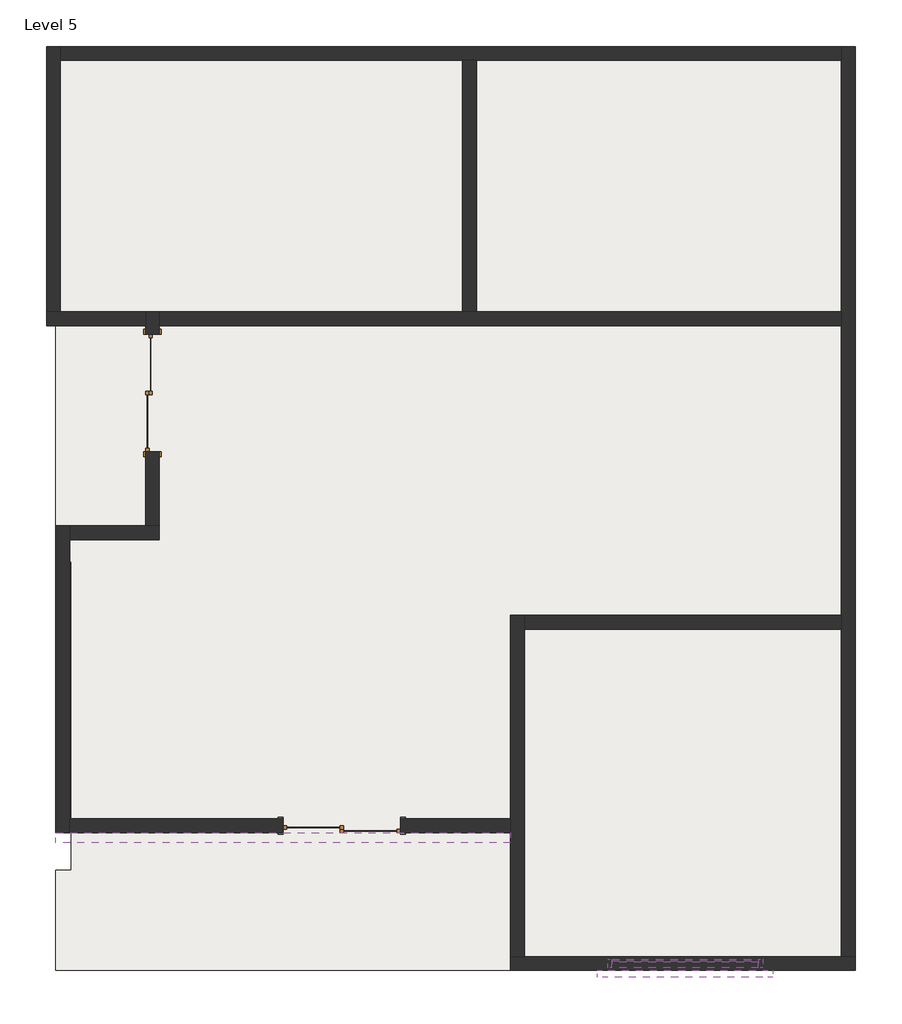
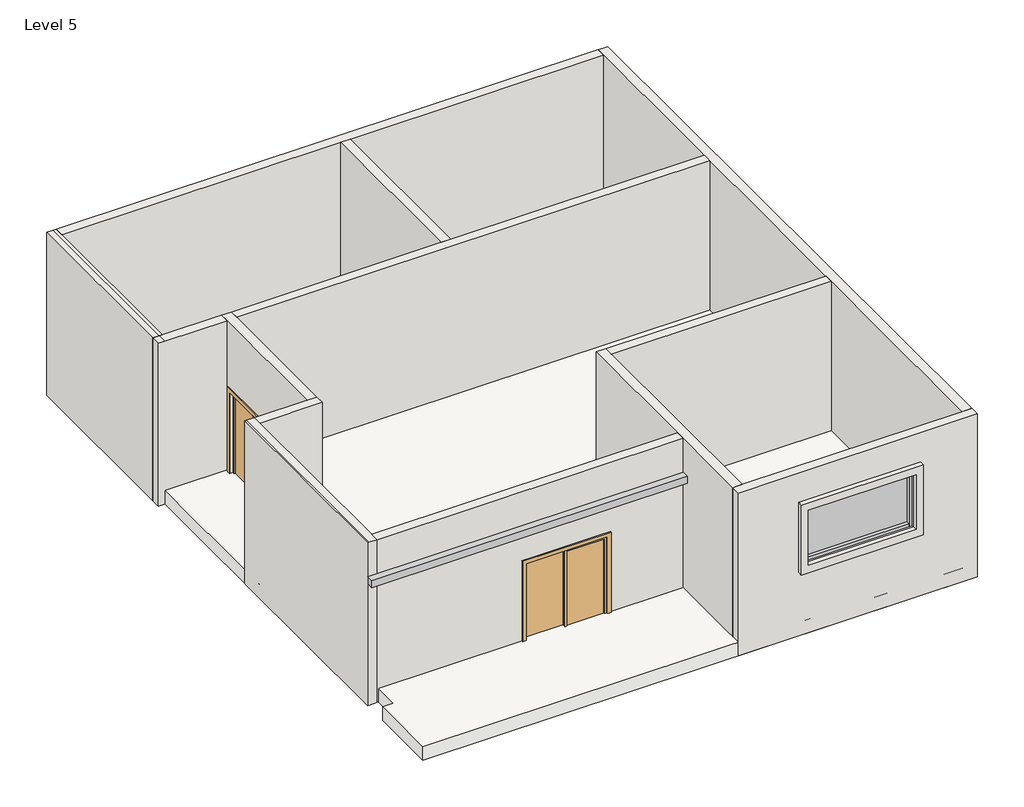
# One storey: 14 walls, 4 members, 2 doors, 1 plate, 1 proxy, 1 roof.
"""IFC4 building model written with IfcOpenShell, lengths in millimetres."""

from ifc_helpers import new_model, si_unit, frame, origin, place, context, project, spatial, polyline, outline, extrude, faceted_brep, transform, mapped, element, save
from components import door_076b30e0, member_3a6679d5, member_c08f7e50, system_panel_glazed_5a0db22b, walls_3_walls_1_a56c50be

model = new_model("IFC4")

# Units and contexts
model_context = context("Model", 3, world=origin())
ifc_project = project(units=[si_unit("LENGTHUNIT", "METRE", prefix="MILLI")], contexts=[model_context])

# Site, building, storey
site = spatial("IfcSite", under=ifc_project)
building = spatial("IfcBuilding", under=site)
storey = spatial("IfcBuildingStorey", under=building, Name="Level 5", Elevation=14630.4)

# Proxy
placement = place(None, origin())
element("IfcBuildingElementProxy", 1, Name="Cornice", ObjectType="Cornice", at=placement, inside=storey, context=model_context, shape_type="SweptSolid", body=[
    extrude(outline(polyline([(-8860.5727738, -2109.6325754), (-8860.5727738, -1957.2325754), (-2155.3436544, -1957.2325754), (-2155.3436544, -2109.6325754), (-8860.5727738, -2109.6325754)])), frame((0.0, 0.0, 17373.6), z_axis=(0.0, 0.0, 1.0), x_axis=(1.0, 0.0, 0.0)), (0.0, 0.0, 1.0), 152.4),
])

# Doors
door_shape = door_076b30e0(model_context)
element("IfcDoor", 2, ObjectType="Door-Double-Sliding : 68\" x 80\"", at=placement, inside=storey, context=model_context, shape_type="MappedRepresentation", body=[
    mapped(door_shape, transform((-7311.1727738, 4519.7674246, 14732.0), x_axis=(0.0, 1.0, 0.0), y_axis=(-1.0, 0.0, 0.0), z_axis=(0.0, 0.0, 1.0))),
])
element("IfcDoor", 3, ObjectType="Door-Double-Sliding : 68\" x 80\"", at=placement, inside=storey, context=model_context, shape_type="MappedRepresentation", body=[
    mapped(door_shape, transform((-4644.5436544, -1728.6325754, 14630.4), x_axis=(-1.0, 0.0, 0.0), y_axis=(0.0, -1.0, 0.0), z_axis=(0.0, 0.0, 1.0))),
])

# Members
member_shape = member_3a6679d5(model_context)
element("IfcMember", 4, ObjectType="Rectangular Mullion : 2.5\" x 5\" rectangular", at=placement, inside=storey, context=model_context, shape_type="MappedRepresentation", body=[
    mapped(member_shape, transform((1560.0533085, -3887.6325754, 16233.9422066), x_axis=(1.0, 0.0, 0.0), y_axis=(0.0, -1.0, 0.0), z_axis=(0.0, 0.0, -1.0))),
])
member_2_shape = member_c08f7e50(model_context)
element("IfcMember", 5, ObjectType="Rectangular Mullion : 2.5\" x 5\" rectangular", at=placement, inside=storey, context=model_context, shape_type="MappedRepresentation", body=[
    mapped(member_2_shape, transform((-662.4466915, -3887.6325754, 16233.9422066), x_axis=(0.0, 0.0, -1.0), y_axis=(0.0, -1.0, 0.0), z_axis=(-1.0, 0.0, 0.0))),
])
element("IfcMember", 6, ObjectType="Rectangular Mullion : 2.5\" x 5\" rectangular", at=placement, inside=storey, context=model_context, shape_type="MappedRepresentation", body=[
    mapped(member_2_shape, transform((1496.5533085, -3887.6325754, 17464.824337), x_axis=(0.0, 0.0, 1.0), y_axis=(0.0, -1.0, 0.0), z_axis=(1.0, 0.0, 0.0))),
])
element("IfcMember", 7, ObjectType="Rectangular Mullion : 2.5\" x 5\" rectangular", at=placement, inside=storey, context=model_context, shape_type="MappedRepresentation", body=[
    mapped(member_shape, transform((-725.9466915, -3887.6325754, 17464.824337), x_axis=(-1.0, 0.0, 0.0), y_axis=(0.0, -1.0, 0.0), z_axis=(0.0, 0.0, 1.0))),
])

# Plate
system_panel_glazed_shape = system_panel_glazed_5a0db22b(model_context)
element("IfcPlate", 8, ObjectType="System Panel : Glazed", at=placement, inside=storey, context=model_context, shape_type="MappedRepresentation", body=[
    mapped(system_panel_glazed_shape, transform((417.0533085, -3887.6325754, 16297.4422066), x_axis=(1.0, 0.0, 0.0), y_axis=(0.0, 1.0, 0.0), z_axis=(0.0, 0.0, 1.0))),
])

# Roof
element("IfcRoof", 9, ObjectType="Generic - 12\"", at=placement, inside=storey, context=model_context, shape_type="SweptSolid", body=[
    extrude(outline(polyline([(-8860.5727738, 9529.9174246), (2924.6563456, 9529.9174246), (2924.6563456, -3989.2325754), (-8860.5727738, -3989.2325754), (-8860.5727738, -2509.6825754), (-8631.9727738, -2509.6825754), (-8631.9727738, 2036.9174246), (-8860.5727738, 2036.9174246), (-8860.5727738, 9529.9174246)])), frame((0.0, 0.0, 14630.4), z_axis=(0.0, 0.0, 1.0), x_axis=(1.0, 0.0, 0.0)), (0.0, 0.0, 1.0), 304.8),
])

# Walls
element("IfcWall", 10, ObjectType="Generic - 8\"", at=placement, inside=storey, context=model_context, shape_type="Brep", body=[
    faceted_brep([(2924.6563456, -3786.0325754, 14630.4), (2721.4563456, -3786.0325754, 14630.4), (-1952.1436544, -3786.0325754, 14630.4), (-2155.3436544, -3786.0325754, 14630.4), (-2155.3436544, -3786.0325754, 18288.0), (-1952.1436544, -3786.0325754, 18288.0), (2721.4563456, -3786.0325754, 18288.0), (2924.6563456, -3786.0325754, 18288.0), (1560.0533085, -3786.0325754, 17464.824337), (-725.9466915, -3786.0325754, 17464.824337), (-725.9466915, -3786.0325754, 16233.9422066), (1560.0533085, -3786.0325754, 16233.9422066), (2924.6563456, -3989.2325754, 14630.4), (2924.6563456, -3989.2325754, 18288.0), (-2155.3436544, -3989.2325754, 18288.0), (-2155.3436544, -3989.2325754, 14630.4), (1560.0533085, -3989.2325754, 17464.824337), (1560.0533085, -3989.2325754, 16233.9422066), (-725.9466915, -3989.2325754, 16233.9422066), (-725.9466915, -3989.2325754, 17464.824337)], [[[0, 1, 2, 3, 4, 5, 6, 7], [8, 9, 10, 11]], [[12, 13, 14, 15], [16, 17, 18, 19]], [[4, 3, 15, 14]], [[0, 7, 13, 12]], [[3, 2, 1, 0, 12, 15]], [[9, 8, 16, 19]], [[10, 9, 19, 18]], [[11, 10, 18, 17]], [[8, 11, 17, 16]], [[7, 6, 5, 4, 14, 13]]]),
])
element("IfcWall", 11, ObjectType="Generic - 8\"", at=placement, inside=storey, context=model_context, shape_type="Brep", body=[
    faceted_brep([(-1952.1436544, -3786.0325754, 14630.4), (-1952.1436544, 1039.9674246, 14630.4), (-1952.1436544, 1243.1674246, 14630.4), (-1952.1436544, 1243.1674246, 18288.0), (-1952.1436544, 1039.9674246, 18288.0), (-1952.1436544, -3786.0325754, 18288.0), (-2155.3436544, -3786.0325754, 14630.4), (-2155.3436544, -3786.0325754, 18288.0), (-2155.3436544, -1957.2325754, 18288.0), (-2155.3436544, -1754.0325754, 18288.0), (-2155.3436544, 1243.1674246, 18288.0), (-2155.3436544, 1243.1674246, 14630.4), (-2155.3436544, -1754.0325754, 14630.4), (-2155.3436544, -1957.2325754, 14630.4)], [[[0, 1, 2, 3, 4, 5]], [[6, 7, 8, 9, 10, 11, 12, 13]], [[2, 1, 0, 6, 13, 12, 11]], [[0, 5, 7, 6]], [[3, 2, 11, 10]], [[5, 4, 3, 10, 9, 8, 7]]]),
])
element("IfcWall", 12, ObjectType="Generic - 8\"", at=placement, inside=storey, context=model_context, shape_type="SweptSolid", body=[
    extrude(outline(polyline([(2716.475018, 1039.9674246), (-1952.1436544, 1039.9674246), (-1952.1436544, 1243.1674246), (2716.475018, 1243.1674246), (2716.475018, 1039.9674246)])), frame((0.0, 0.0, 14630.4), z_axis=(0.0, 0.0, 1.0), x_axis=(1.0, 0.0, 0.0)), (0.0, 0.0, 1.0), 3657.6),
])
element("IfcWall", 13, ObjectType="Generic - 8\"", at=placement, inside=storey, context=model_context, shape_type="SweptSolid", body=[
    extrude(outline(polyline([(2924.6563456, 9625.1674246), (2924.6563456, -3786.0325754), (2721.4563456, -3786.0325754), (2721.4563456, 9625.1674246), (2924.6563456, 9625.1674246)])), frame((0.0, 0.0, 14630.4), z_axis=(0.0, 0.0, 1.0), x_axis=(1.0, 0.0, 0.0)), (0.0, 0.0, 1.0), 3657.6),
])
element("IfcWall", 14, ObjectType="Generic - 8\"", at=placement, inside=storey, context=model_context, shape_type="Brep", body=[
    faceted_brep([(-8657.3727738, -1957.2325754, 14630.4), (-8657.3727738, -1754.0325754, 14630.4), (-8657.3727738, 2360.7674246, 14630.4), (-8657.3727738, 2563.9674246, 14630.4), (-8657.3727738, 2563.9674246, 18288.0), (-8657.3727738, 2360.7674246, 18288.0), (-8657.3727738, -1754.0325754, 18288.0), (-8657.3727738, -1957.2325754, 18288.0), (-8860.5727738, -1957.2325754, 14630.4), (-8860.5727738, -1957.2325754, 18288.0), (-8860.5727738, 2563.9674246, 18288.0), (-8860.5727738, 2563.9674246, 14630.4), (-8835.1727738, 2563.9674246, 18288.0), (-8835.1727738, -1957.2325754, 18288.0)], [[[0, 1, 2, 3, 4, 5, 6, 7]], [[8, 9, 10, 11]], [[3, 2, 1, 0, 8, 11]], [[4, 3, 11, 10, 12]], [[0, 7, 13, 9, 8]], [[12, 10, 9, 13]], [[7, 6, 5, 4, 12, 13]]]),
])
element("IfcWall", 15, ObjectType="Generic - 8\"", at=placement, inside=storey, context=model_context, shape_type="Brep", body=[
    faceted_brep([(-8657.3727738, 2360.7674246, 14630.4), (-7336.5727738, 2360.7674246, 14630.4), (-7336.5727738, 2360.7674246, 18288.0), (-8657.3727738, 2360.7674246, 18288.0), (-8657.3727738, 2563.9674246, 14630.4), (-8657.3727738, 2563.9674246, 18288.0), (-7539.7727738, 2563.9674246, 18288.0), (-7336.5727738, 2563.9674246, 18288.0), (-7336.5727738, 2563.9674246, 14630.4), (-7539.7727738, 2563.9674246, 14630.4)], [[[0, 1, 2, 3]], [[4, 5, 6, 7, 8, 9]], [[1, 0, 4, 9, 8]], [[0, 3, 5, 4]], [[2, 1, 8, 7]], [[3, 2, 7, 6, 5]]]),
])
element("IfcWall", 16, ObjectType="Generic - 8\"", at=placement, inside=storey, context=model_context, shape_type="Brep", body=[
    faceted_brep([(-7336.5727738, 2563.9674246, 14630.4), (-7336.5727738, 5510.3674246, 14630.4), (-7336.5727738, 5713.5674246, 14630.4), (-7336.5727738, 5713.5674246, 18288.0), (-7336.5727738, 5510.3674246, 18288.0), (-7336.5727738, 2563.9674246, 18288.0), (-7336.5727738, 3656.1674246, 16764.0), (-7336.5727738, 5383.3674246, 16764.0), (-7336.5727738, 5383.3674246, 14732.0), (-7336.5727738, 3656.1674246, 14732.0), (-7539.7727738, 2563.9674246, 14630.4), (-7539.7727738, 2563.9674246, 18288.0), (-7539.7727738, 5510.3674246, 18288.0), (-7539.7727738, 5713.5674246, 18288.0), (-7539.7727738, 5713.5674246, 14630.4), (-7539.7727738, 5510.3674246, 14630.4), (-7539.7727738, 3656.1674246, 16764.0), (-7539.7727738, 3656.1674246, 14732.0), (-7539.7727738, 5383.3674246, 14732.0), (-7539.7727738, 5383.3674246, 16764.0)], [[[0, 1, 2, 3, 4, 5], [6, 7, 8, 9]], [[10, 11, 12, 13, 14, 15], [16, 17, 18, 19]], [[2, 1, 0, 10, 15, 14]], [[0, 5, 11, 10]], [[3, 2, 14, 13]], [[5, 4, 3, 13, 12, 11]], [[17, 16, 6, 9]], [[18, 17, 9, 8]], [[19, 18, 8, 7]], [[16, 19, 7, 6]]]),
])
element("IfcWall", 17, ObjectType="Generic - 8\"", at=placement, inside=storey, context=model_context, shape_type="Brep", body=[
    faceted_brep([(-7539.7727738, 5713.5674246, 14630.4), (-8796.074982, 5713.5674246, 14630.4), (-8999.274982, 5713.5674246, 14630.4), (-8999.274982, 5713.5674246, 18288.0), (-8860.5727738, 5713.5674246, 18288.0), (-8796.074982, 5713.5674246, 18288.0), (-7539.7727738, 5713.5674246, 18288.0), (-7539.7727738, 5510.3674246, 14630.4), (-7539.7727738, 5510.3674246, 18288.0), (-8860.5727738, 5510.3674246, 18288.0), (-8999.274982, 5510.3674246, 18288.0), (-8999.274982, 5510.3674246, 14630.4)], [[[0, 1, 2, 3, 4, 5, 6]], [[7, 8, 9, 10, 11]], [[2, 1, 0, 7, 11]], [[0, 6, 8, 7]], [[3, 2, 11, 10]], [[4, 3, 10, 9]], [[6, 5, 4, 9, 8]]]),
])
element("IfcWall", 18, ObjectType="Generic - 8\"", at=placement, inside=storey, context=model_context, shape_type="Brep", body=[
    faceted_brep([(-8796.074982, 5713.5674246, 14630.4), (-8796.074982, 9421.9674246, 14630.4), (-8796.074982, 9625.1674246, 14630.4), (-8796.074982, 9625.1674246, 18288.0), (-8796.074982, 9421.9674246, 18288.0), (-8796.074982, 5713.5674246, 18288.0), (-8999.274982, 5713.5674246, 14630.4), (-8999.274982, 5713.5674246, 18288.0), (-8999.274982, 9625.1674246, 18288.0), (-8999.274982, 9625.1674246, 14630.4), (-8860.5727738, 5713.5674246, 18288.0), (-8860.5727738, 9625.1674246, 18288.0)], [[[0, 1, 2, 3, 4, 5]], [[6, 7, 8, 9]], [[2, 1, 0, 6, 9]], [[0, 5, 10, 7, 6]], [[3, 2, 9, 8, 11]], [[5, 4, 3, 11, 10]], [[11, 8, 7, 10]]]),
])
element("IfcWall", 19, ObjectType="Generic - 8\"", at=placement, inside=storey, context=model_context, shape_type="Brep", body=[
    faceted_brep([(-8796.074982, 9421.9674246, 14630.4), (-2866.5436544, 9421.9674246, 14630.4), (-2663.3436544, 9421.9674246, 14630.4), (2716.475018, 9421.9674246, 14630.4), (2716.475018, 9421.9674246, 18288.0), (-2663.3436544, 9421.9674246, 18288.0), (-2866.5436544, 9421.9674246, 18288.0), (-8796.074982, 9421.9674246, 18288.0), (-8796.074982, 9625.1674246, 14630.4), (-8796.074982, 9625.1674246, 18288.0), (2716.475018, 9625.1674246, 18288.0), (2716.475018, 9625.1674246, 14630.4)], [[[0, 1, 2, 3, 4, 5, 6, 7]], [[8, 9, 10, 11]], [[3, 2, 1, 0, 8, 11]], [[4, 3, 11, 10]], [[0, 7, 9, 8]], [[7, 6, 5, 4, 10, 9]]]),
])
element("IfcWall", 20, ObjectType="Generic - 8\"", at=placement, inside=storey, context=model_context, shape_type="Brep", body=[
    faceted_brep([(-7336.5727738, 5510.3674246, 14630.4), (2716.475018, 5510.3674246, 14630.4), (2716.475018, 5510.3674246, 18288.0), (-7336.5727738, 5510.3674246, 18288.0), (-7336.5727738, 5713.5674246, 14630.4), (-7336.5727738, 5713.5674246, 18288.0), (-2866.5436544, 5713.5674246, 18288.0), (-2663.3436544, 5713.5674246, 18288.0), (2716.475018, 5713.5674246, 18288.0), (2716.475018, 5713.5674246, 14630.4), (-2663.3436544, 5713.5674246, 14630.4), (-2866.5436544, 5713.5674246, 14630.4)], [[[0, 1, 2, 3]], [[4, 5, 6, 7, 8, 9, 10, 11]], [[1, 0, 4, 11, 10, 9]], [[2, 1, 9, 8]], [[0, 3, 5, 4]], [[3, 2, 8, 7, 6, 5]]]),
])
element("IfcWall", 21, ObjectType="Generic - 8\"", at=placement, inside=storey, context=model_context, shape_type="SweptSolid", body=[
    extrude(outline(polyline([(-2663.3436544, 9421.9674246), (-2663.3436544, 5713.5674246), (-2866.5436544, 5713.5674246), (-2866.5436544, 9421.9674246), (-2663.3436544, 9421.9674246)])), frame((0.0, 0.0, 14630.4), z_axis=(0.0, 0.0, 1.0), x_axis=(1.0, 0.0, 0.0)), (0.0, 0.0, 1.0), 3657.6),
])
element("IfcWall", 22, ObjectType="Generic - 8\"", at=placement, inside=storey, context=model_context, shape_type="SweptSolid", body=[
    extrude(outline(polyline([(14630.4, -8657.3727738), (14630.4, -5508.1436544), (16662.4, -5508.1436544), (16662.4, -3780.9436544), (14630.4, -3780.9436544), (14630.4, -2155.3436544), (18288.0, -2155.3436544), (18288.0, -8657.3727738), (14630.4, -8657.3727738)])), frame((0.0, -1957.2325754, 0.0), z_axis=(0.0, 1.0, 0.0), x_axis=(0.0, 0.0, 1.0)), (0.0, 0.0, 1.0), 203.2),
])
walls_3_walls_1_shape = walls_3_walls_1_a56c50be(model_context)
element("IfcWall", 23, ObjectType="Walls 3 : Walls 1", at=placement, inside=storey, context=model_context, shape_type="MappedRepresentation", body=[
    mapped(walls_3_walls_1_shape, transform((0.0, 0.0, 0.0), x_axis=(1.0, 0.0, 0.0), y_axis=(0.0, 1.0, 0.0), z_axis=(0.0, 0.0, 1.0))),
])

save(model, "model.ifc")

# Revit data of these elements
# Type "Door-Double-Sliding : 68\" x 80\""
#   Type Mark = "10"
#   Construction Type Id = "opn-d45"
#   Assembly Code = "C1020"
#   Analytic Construction = "Wood frame, double glass door "
#   Thickness = 0' - 2"
#   Thermal Resistance (R) = 1.8150 (h·ft²·°F)/BTU
#   Heat Transfer Coefficient (U) = 0.5510 BTU/(h·ft²·°F)
#   Height = 6' - 8"
#   Rail Width = 0' - 2"
#   Stiles = 0' - 2"
#   Trim Projection Ext = 0' - 1"
#   Trim Projection Int = 0' - 1"
#   Trim Width = 0' - 3"
#   Width = 5' - 8"
#   Define Thermal Properties by = 1
#   Glazing = Glass
#   Panel Material = Wood - Birch - Solid Stained Light Low Gloss
#   Trim Material = Paint - Sienna
#   Visual Light Transmittance = 0
#   Solar Heat Gain Coefficient = 0
#   Function = (empty or 0)
#   Wall Closure = (empty or 0)
# Type "Rectangular Mullion : 2.5\" x 5\" rectangular"
#   built-in parameter 1007304 = 0.416667 (stored number, unit not read)
#   built-in parameter 1007301 = 0.104167 (stored number, unit not read)
#   built-in parameter 1007300 = 0.104167 (stored number, unit not read)
# Type "System Panel : Glazed"
#   Construction Type Id = "GSP4R"
#   Analytic Construction = "1/8 in Pilkington single glazing"
#   Visual Light Transmittance = 0.9
#   Solar Heat Gain Coefficient = 0.86
#   Heat Transfer Coefficient (U) = 1.18115 BTU/(h·ft²·°F)
# Type "Generic - 12\""
#   Assembly Code = "B1020"
#   Layers, outside or top first: 1' - 0" no material (function 1)
# Type "Generic - 8\""
#   Assembly Code = "B2010"
#   Layers, outside or top first: 0' - 8" no material (function 1)
# Element 1 (IfcBuildingElementProxy, "Cornice")
#   Phase Created = New Construction
#   Materials on its faces: "Default Wall"
# Elements 2, 3 (IfcDoor, "Door-Double-Sliding : 68\" x 80\"")
#   Phase Created = New Construction
#   Materials on its faces: "Paint - Sienna", "Wood - Birch - Solid Stained Light Low Gloss", "Glass"
# Elements 4, 5, 6, 7 (IfcMember, "Rectangular Mullion : 2.5\" x 5\" rectangular")
#   Phase Created = New Construction
#   Materials on its faces: "Aluminum"
# Element 8 (IfcPlate, "System Panel : Glazed")
#   Phase Created = New Construction
#   Materials on its faces: "Glass"
# Element 9 (IfcRoof, "Generic - 12\"")
#   built-in parameter 1001705 = 49 (stored number, unit not read)
#   built-in parameter 1001710 = 33615
#   Phase Created = New Construction
#   Materials on its faces: "Default Roof"
# Elements 10, 11, 12, 13, 14, 15, 16, 17, 18, 19, 20, 21, 22 (IfcWall, "Generic - 8\"")
#   Top Offset = 0' - 0"
#   Base Offset = 0' - 0"
#   Unconnected Height = 12' - 0"
#   wall height = 12' - 0"
#   Phase Created = New Construction
#   Base Constraint = Level 5
#   Materials on its faces: "Default Wall"
# Element 23 (IfcWall, "Walls 3 : Walls 1")
#   Phase Created = New Construction
#   Materials on its faces: "Default Wall"
# Materials
#   "Glass": class "Glass", colour RGB 0 128 192, transparency 0.75, Description = "Soda Lime Glass", Cost = 0
#   "Wood - Birch - Solid Stained Light Low Gloss": class "Wood", colour RGB 210 159 95, transparency 0, Cost = 0
#   "Paint - Sienna": colour RGB 118 70 51, transparency 0, Cost = 0
#   "Default Wall": colour RGB 128 128 128, transparency 0
#   "Aluminum": class "Metal", colour RGB 247 247 247, transparency 0, Description = "Aluminum 6061", Cost = 0
#   "Default Roof": colour RGB 88 101 114, transparency 0
